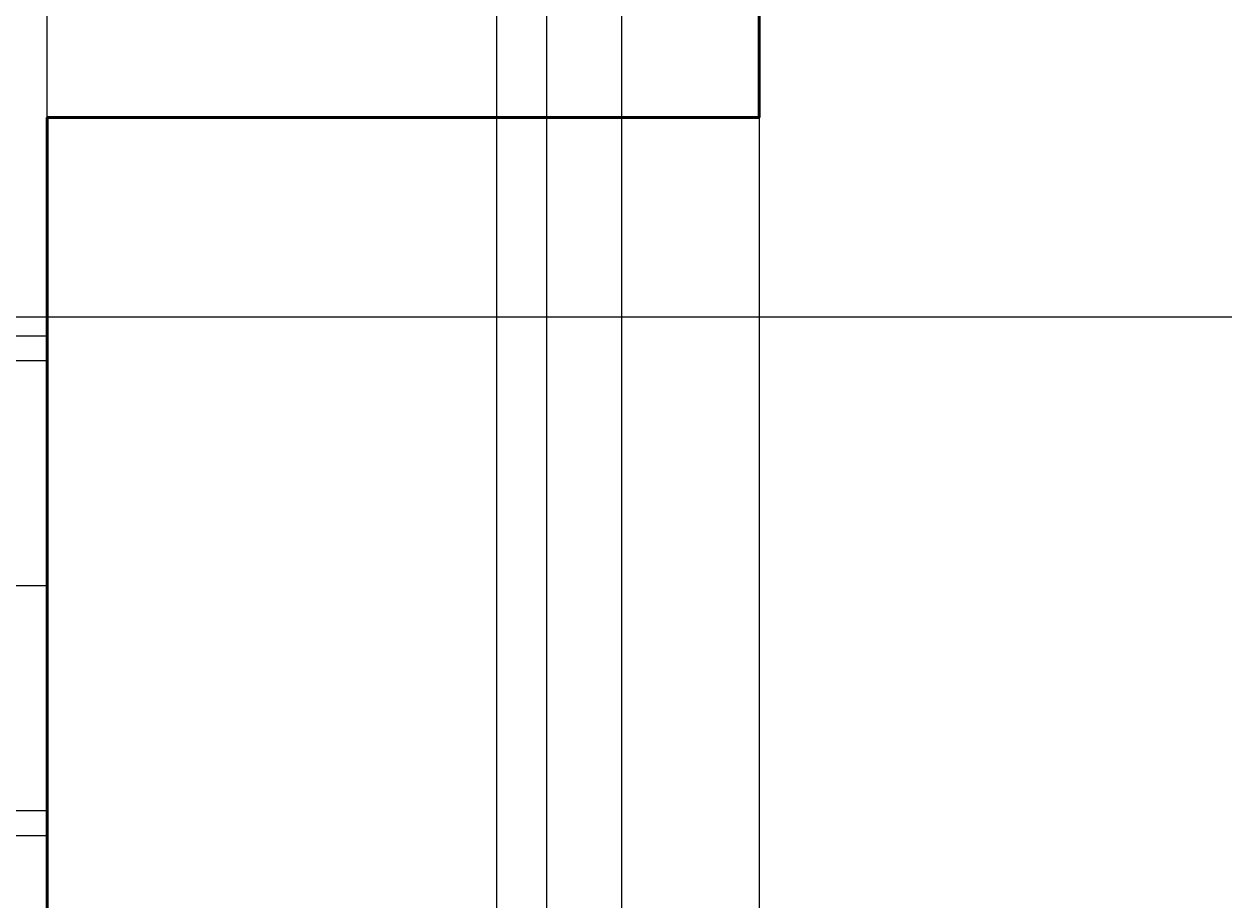
# Model space of a CAD drawing. Units: inches. Extents: x 37 to 824, y -700 to 234.
# Tile 43 of 77: x 168 to 264, y -75 to -4. Entities that reach past the tile are written whole.
import ezdxf

# ---------------------------------------------------------------- set-up
doc = ezdxf.new("R2010")
doc.units = ezdxf.units.IN
doc.header["$MEASUREMENT"] = 0
for name, color, linetype, lineweight in [('A-ANNO-DIMS', 2, 'Continuous', 18), ('A-GLAZ', 4, 'Continuous', 25), ('A-WALL', 2, 'Continuous', 50)]:
    doc.layers.add(name, color=color, linetype=linetype, lineweight=lineweight)
doc.styles.get("Standard").update_dxf_attribs({"font": 'arial.ttf'})
doc.dimstyles.get("Standard").update_dxf_attribs({"dimtxt": 0.18, "dimasz": 0.18, "dimexe": 0.18, "dimexo": 0.0625, "dimgap": 0.09, "dimtad": 0, "dimtih": 1, "dimtoh": 1, "dimdec": 1, "dimzin": 0, "dimdsep": 46, "dimlunit": 4, "dimtxsty": 'Standard', "dimcen": 0.09, "dimadec": 0, "dimazin": 0, "dimtfac": 1, "dimtdec": 1, "dimtofl": 0, "dimtmove": 0, "dimatfit": 3, "dimfxl": 1, "dimtolj": 1, "dimtzin": 0, "dimarcsym": 0})

# ---------------------------------------------------------------- blocks, each defined once
blk = doc.blocks.new('WIN-900')
for p, q in [((0, 9), (0, 0)), ((2, 9), (2, 0)), ((20, 9), (20, 0)), ((38, 9), (38, 0)), ((40, 9), (40, 0)), ((38, 5.5), (2, 5.5)), ((38, 3.5), (2, 3.5))]:
    blk.add_line(p, q)
blk = doc.blocks.new('*D62')
at = {"layer": 'A-ANNO-DIMS', "color": 0, "lineweight": -2, "ltscale": 0.5, "transparency": 16777216}
for p, q in [((419.015, 6.09), (78.159, 6.09)), ((78.339, 5.91), (78.339, -10.728)), ((78.339, -27.73), (78.339, -11.091)), ((419.015, -27.91), (78.159, -27.91))]:
    blk.add_line(p, q, dxfattribs=at)
at = {"layer": 'A-ANNO-DIMS', "color": 0, "ltscale": 0.5, "transparency": 16777216}
for points in [[(78.309, 5.91), (78.369, 5.91), (78.339, 6.09)], [(78.309, -27.73), (78.369, -27.73), (78.339, -27.91)]]:
    blk.add_solid(points, dxfattribs=at)
at = {"layer": 'Defpoints', "color": 0, "ltscale": 0.5, "transparency": 16777216}
for p in [(419.077, 6.09), (78.339, -27.91), (419.077, -27.91)]:
    blk.add_point(p, dxfattribs=at)
at = {"layer": 'A-ANNO-DIMS', "color": 0, "ltscale": 0.5, "transparency": 16777216, "insert": (78.339, -10.91), "char_height": 0.18, "attachment_point": 5}
blk.add_mtext('\\A1;2\'-10"', dxfattribs=at)
blk = doc.blocks.new('*D77')
at = {"layer": 'A-ANNO-DIMS', "color": 0, "lineweight": -2, "ltscale": 0.5, "transparency": 16777216}
for p, q in [((227.077, 45.5), (227.077, -400.406)), ((290.077, 15.028), (290.077, -400.406)), ((227.257, -400.226), (258.248, -400.226)), ((289.897, -400.226), (258.906, -400.226))]:
    blk.add_line(p, q, dxfattribs=at)
at = {"layer": 'A-ANNO-DIMS', "color": 0, "ltscale": 0.5, "transparency": 16777216}
for points in [[(227.257, -400.196), (227.257, -400.256), (227.077, -400.226)], [(289.897, -400.196), (289.897, -400.256), (290.077, -400.226)]]:
    blk.add_solid(points, dxfattribs=at)
at = {"layer": 'Defpoints', "color": 0, "ltscale": 0.5, "transparency": 16777216}
for p in [(227.077, 45.563), (290.077, 15.09), (290.077, -400.226)]:
    blk.add_point(p, dxfattribs=at)
at = {"layer": 'A-ANNO-DIMS', "color": 0, "ltscale": 0.5, "transparency": 16777216, "insert": (258.577, -400.226), "char_height": 0.18, "attachment_point": 5}
blk.add_mtext('\\A1;5\'-3"', dxfattribs=at)
blk = doc.blocks.new('*D84')
at = {"layer": 'A-ANNO-DIMS', "color": 0, "lineweight": -2, "ltscale": 0.5, "transparency": 16777216}
for p, q in [((170.077, -265.847), (170.077, 234.17)), ((170.257, 233.99), (189.748, 233.99)), ((209.897, 233.99), (190.406, 233.99)), ((210.077, -265.847), (210.077, 234.17))]:
    blk.add_line(p, q, dxfattribs=at)
at = {"layer": 'A-ANNO-DIMS', "color": 0, "ltscale": 0.5, "transparency": 16777216}
for points in [[(170.257, 234.02), (170.257, 233.96), (170.077, 233.99)], [(209.897, 234.02), (209.897, 233.96), (210.077, 233.99)]]:
    blk.add_solid(points, dxfattribs=at)
at = {"layer": 'Defpoints', "color": 0, "ltscale": 0.5, "transparency": 16777216}
for p in [(210.077, 233.99), (170.077, -265.91), (210.077, -265.91)]:
    blk.add_point(p, dxfattribs=at)
at = {"layer": 'A-ANNO-DIMS', "color": 0, "ltscale": 0.5, "transparency": 16777216, "insert": (190.077, 233.99), "char_height": 0.18, "attachment_point": 5}
blk.add_mtext('\\A1;3\'-4"', dxfattribs=at)
blk = doc.blocks.new('*D85')
at = {"layer": 'A-ANNO-DIMS', "color": 0, "lineweight": -2, "ltscale": 0.5, "transparency": 16777216}
for p, q in [((170.077, -356.847), (170.077, 234.17)), ((170.257, 233.99), (187.748, 233.99)), ((205.897, 233.99), (188.406, 233.99)), ((206.077, -356.847), (206.077, 234.17))]:
    blk.add_line(p, q, dxfattribs=at)
at = {"layer": 'A-ANNO-DIMS', "color": 0, "ltscale": 0.5, "transparency": 16777216}
for points in [[(170.257, 234.02), (170.257, 233.96), (170.077, 233.99)], [(205.897, 234.02), (205.897, 233.96), (206.077, 233.99)]]:
    blk.add_solid(points, dxfattribs=at)
at = {"layer": 'Defpoints', "color": 0, "ltscale": 0.5, "transparency": 16777216}
for p in [(206.077, 233.99), (170.077, -356.91), (206.077, -356.91)]:
    blk.add_point(p, dxfattribs=at)
at = {"layer": 'A-ANNO-DIMS', "color": 0, "ltscale": 0.5, "transparency": 16777216, "insert": (188.077, 233.99), "char_height": 0.18, "attachment_point": 5}
blk.add_mtext('\\A1;3\'-0"', dxfattribs=at)
blk = doc.blocks.new('*D86')
at = {"layer": 'A-ANNO-DIMS', "color": 0, "lineweight": -2, "ltscale": 0.5, "transparency": 16777216}
for p, q in [((206.077, -356.847), (206.077, 234.17)), ((206.257, 233.99), (210.678, 233.99)), ((215.897, 233.99), (211.476, 233.99)), ((216.077, -356.847), (216.077, 234.17))]:
    blk.add_line(p, q, dxfattribs=at)
at = {"layer": 'A-ANNO-DIMS', "color": 0, "ltscale": 0.5, "transparency": 16777216}
for points in [[(206.257, 234.02), (206.257, 233.96), (206.077, 233.99)], [(215.897, 234.02), (215.897, 233.96), (216.077, 233.99)]]:
    blk.add_solid(points, dxfattribs=at)
at = {"layer": 'Defpoints', "color": 0, "ltscale": 0.5, "transparency": 16777216}
for p in [(216.077, 233.99), (206.077, -356.91), (216.077, -356.91)]:
    blk.add_point(p, dxfattribs=at)
at = {"layer": 'A-ANNO-DIMS', "color": 0, "ltscale": 0.5, "transparency": 16777216, "insert": (211.077, 233.99), "char_height": 0.18, "attachment_point": 5}
blk.add_mtext('\\A1;0\'-10"', dxfattribs=at)
blk = doc.blocks.new('*D87')
at = {"layer": 'A-ANNO-DIMS', "color": 0, "lineweight": -2, "ltscale": 0.5, "transparency": 16777216}
for p, q in [((216.077, -356.847), (216.077, 234.17)), ((216.257, 233.99), (255.747, 233.99)), ((295.897, 233.99), (256.407, 233.99)), ((296.077, -356.847), (296.077, 234.17))]:
    blk.add_line(p, q, dxfattribs=at)
at = {"layer": 'A-ANNO-DIMS', "color": 0, "ltscale": 0.5, "transparency": 16777216}
for points in [[(216.257, 234.02), (216.257, 233.96), (216.077, 233.99)], [(295.897, 234.02), (295.897, 233.96), (296.077, 233.99)]]:
    blk.add_solid(points, dxfattribs=at)
at = {"layer": 'Defpoints', "color": 0, "ltscale": 0.5, "transparency": 16777216}
for p in [(296.077, 233.99), (216.077, -356.91), (296.077, -356.91)]:
    blk.add_point(p, dxfattribs=at)
at = {"layer": 'A-ANNO-DIMS', "color": 0, "ltscale": 0.5, "transparency": 16777216, "insert": (256.077, 233.99), "char_height": 0.18, "attachment_point": 5}
blk.add_mtext('\\A1;6\'-8"', dxfattribs=at)

msp = doc.modelspace()

# ---------------------------------------------------------------- linework, layer by layer
at = {"layer": 'A-WALL'}
for p, q in [((227.077, -11.91), (227.077, 45.826)), ((170.077, -11.91), (227.077, -11.91)), ((170.077, -11.91), (170.077, -158.91))]:
    msp.add_line(p, q, dxfattribs=at)

# ---------------------------------------------------------------- block references
at = {"layer": 'A-GLAZ', "rotation": 269.9999999999999}
msp.add_blockref('WIN-900', (161.077, -29.409), dxfattribs=at)

# ---------------------------------------------------------------- dimensions: what is measured, and where the dimension line sits
at = {"layer": 'A-ANNO-DIMS', "ltscale": 0.5}
for base, p1, p2, picture, middle in [((210.077, 233.99), (170.077, -265.91), (210.077, -265.91), '*D84', (190.077, 233.99)), ((206.077, 233.99), (170.077, -356.91), (206.077, -356.91), '*D85', (188.077, 233.99)), ((216.077, 233.99), (206.077, -356.91), (216.077, -356.91), '*D86', (211.077, 233.99)), ((296.077, 233.99), (216.077, -356.91), (296.077, -356.91), '*D87', (256.077, 233.99)), ((290.077, -400.226), (227.077, 45.563), (290.077, 15.09), '*D77', (258.577, -400.226))]:
    dim = msp.add_linear_dim(base=base, p1=p1, p2=p2, dimstyle='Standard', override={"dimdec": 1, "dimlfac": 1, "dimrnd": 0, "dimzin": 1, "dimdsep": 46, "dimlunit": 4, "dimfrac": 2}, dxfattribs=at)
    dim.commit()
    dim.dimension.update_dxf_attribs({"geometry": picture, "text_midpoint": middle})
dim = msp.add_linear_dim(base=(78.339, -27.91), p1=(419.077, 6.09), p2=(419.077, -27.91), angle=90, dimstyle='Standard', override={"dimdec": 1, "dimlfac": 1, "dimrnd": 0, "dimzin": 1, "dimdsep": 46, "dimlunit": 4, "dimfrac": 2}, dxfattribs=at)
dim.commit()
dim.dimension.update_dxf_attribs({"geometry": '*D62', "text_midpoint": (78.339, -10.91)})

doc.saveas('drawing.dxf')
